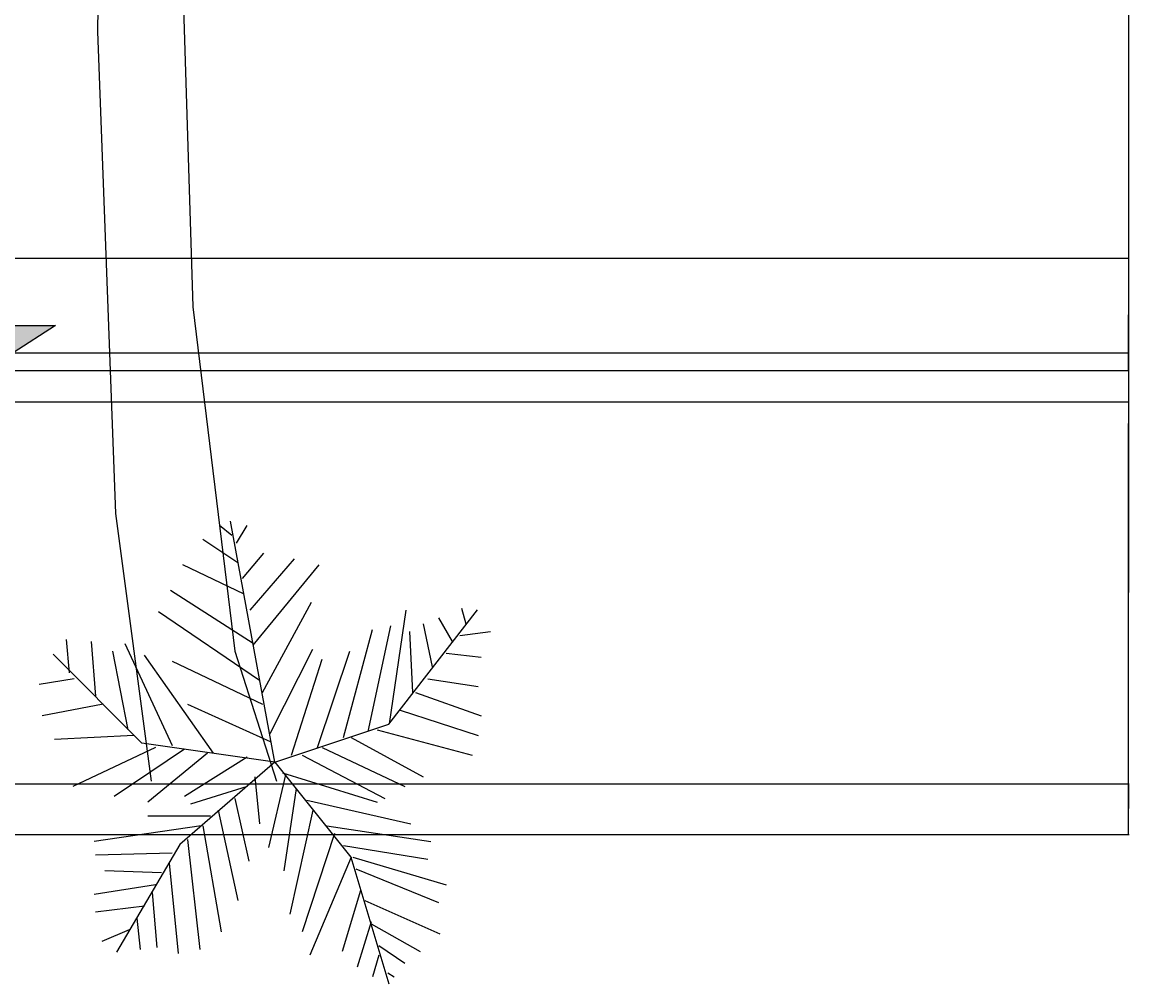
# Model space of a CAD drawing. Units: inches. Extents: x 484 to 1264, y 95 to 991.
# Tile 6 of 8: x 1002 to 1264, y 271 to 499. Entities that reach past the tile are written whole.
import ezdxf

# ---------------------------------------------------------------- set-up
doc = ezdxf.new("R2010")
doc.units = ezdxf.units.IN
doc.header["$MEASUREMENT"] = 0
doc.layers.add('A-ANNO-DIMS', color=2, linetype='Continuous', lineweight=18)
doc.layers.add('L-FENC', color=7, linetype='Continuous', lineweight=25)
doc.layers.add('A-ELEV-TRIM-PATT', color=40, linetype='Continuous', lineweight=13, true_color=0xe7c208)
doc.layers.add('TREES', color=92, linetype='Continuous')
doc.styles.get("Standard").update_dxf_attribs({"font": 'arial.ttf'})
doc.dimstyles.get("Standard").update_dxf_attribs({"dimtxt": 0.18, "dimasz": 0.18, "dimexe": 0.18, "dimexo": 0.0625, "dimgap": 0.09, "dimtad": 0, "dimtih": 1, "dimtoh": 1, "dimdec": 4, "dimzin": 0, "dimdsep": 46, "dimtxsty": 'Standard', "dimcen": 0.09, "dimadec": 0, "dimazin": 0, "dimtfac": 1, "dimtdec": 4, "dimtofl": 0, "dimtmove": 0, "dimatfit": 3, "dimfxl": 1, "dimtolj": 1, "dimtzin": 0, "dimarcsym": 0})

# ---------------------------------------------------------------- blocks, each defined once
blk = doc.blocks.new('*U2')
for p, q in [((-10.186, 53.64), (-13.084, 55.962)), ((0, 0), (-10.5, 57)), ((-9.099, 51.782), (-6.563, 55.962)), ((-8.737, 47.138), (-17.069, 52.711)), ((-7.65, 43.423), (-2.578, 49.46)), ((-5.839, 35.992), (4.667, 48.067)), ((-7.288, 39.707), (-21.778, 46.673)), ((-5.114, 27.632), (10.463, 46.673)), ((-5.114, 28.097), (-24.676, 40.636)), ((-2.941, 16.486), (8.652, 37.85)), ((-3.665, 19.273), (-27.574, 35.527)), ((27, 9), (48, 36)), ((27.127, 9.056), (31.112, 35.992)), ((38.719, 34.134), (41.979, 28.561)), ((44.153, 36.456), (45.239, 32.741)), ((22.055, 7.198), (27.489, 32.277)), ((35.096, 32.741), (37.27, 22.524)), ((-48.585, 21.131), (-49.309, 29.026)), ((16.259, 5.805), (23.142, 31.348)), ((31.836, 30.883), (32.561, 16.486)), ((43.791, 29.954), (51.036, 30.883)), ((-43.513, 28.561), (-42.427, 15.558)), ((-38.442, 26.239), (-34.819, 7.663)), ((-35.544, 28.097), (-24.314, 3.947)), ((-1.129, 6.734), (9.014, 26.704)), ((10.101, 3.483), (17.708, 26.239)), ((-31.5, 4.5), (-52.5, 25.5)), ((-14.533, 2.09), (-30.834, 25.31)), ((-24.314, 23.917), (-2.941, 13.7)), ((3.942, 1.625), (11.187, 24.381)), ((40.53, 25.775), (48.862, 24.846)), ((-47.498, 19.737), (-55.83, 18.344)), ((36.183, 19.737), (48.137, 17.88)), ((33.285, 16.486), (48.862, 10.913)), ((-40.615, 13.7), (-55.105, 10.913)), ((-20.691, 13.7), (-1.129, 4.876)), ((29.662, 12.307), (48.137, 6.269)), ((0, 0), (27, 9)), ((-33.37, 6.269), (-52.207, 5.34)), ((18.07, 5.805), (35.096, -3.483)), ((24.229, 7.663), (46.688, 1.625)), ((-28.299, 3.483), (-47.86, -5.805)), ((-21.416, 3.018), (-38.079, -8.128)), ((0, 0), (-31.5, 4.5)), ((11.187, 3.483), (30.749, -5.805)), ((-15.982, 2.09), (-30.11, -9.521)), ((0, 0), (-22.5, -19.5)), ((-6.563, 1.161), (-21.416, -8.128)), ((0, 0), (18, -22.5)), ((6.478, 1.625), (26.04, -8.592)), ((1.769, -2.555), (24.229, -9.521)), ((-4.752, -3.483), (-3.665, -14.629)), ((2.493, -3.019), (-1.491, -20.202)), ((-6.563, -5.805), (-19.967, -9.985)), ((5.029, -6.27), (2.131, -25.775)), ((-9.461, -8.592), (-6.201, -23.453)), ((7.565, -9.056), (32.198, -14.629)), ((-15.257, -12.772), (-30.11, -12.772)), ((-13.446, -11.378), (-8.737, -32.741)), ((9.014, -11.378), (3.58, -35.992)), ((-17.431, -15.094), (-42.789, -18.809)), ((-17.069, -15.094), (-12.721, -40.172)), ((12.274, -15.094), (36.907, -18.809)), ((-20.691, -18.345), (-17.793, -44.352)), ((14.085, -16.951), (6.478, -40.172)), ((-22.5, -19.5), (-37.5, -45)), ((16.259, -19.738), (36.183, -22.989)), ((-24.314, -21.596), (-42.427, -22.06)), ((18.07, -22.524), (8.289, -45.745)), ((18, -22.5), (27, -52.5)), ((18.433, -22.524), (40.53, -29.026)), ((-26.849, -26.24), (-40.253, -25.775)), ((-25.038, -23.918), (-22.865, -45.281)), ((19.157, -25.311), (38.719, -33.206)), ((-28.299, -29.026), (-42.789, -31.348)), ((-29.023, -30.884), (-27.936, -43.887)), ((20.244, -30.419), (15.897, -44.816)), ((21.331, -32.741), (39.081, -40.636)), ((-30.834, -34.135), (-42.427, -35.528)), ((-32.646, -36.921), (-31.921, -44.352)), ((22.78, -37.85), (19.519, -48.532)), ((22.78, -38.314), (34.372, -44.816)), ((-34.457, -39.708), (-40.978, -42.494)), ((24.591, -43.423), (30.749, -47.603)), ((24.591, -45.745), (23.142, -50.854)), ((26.764, -49.925), (28.213, -50.854))]:
    blk.add_line(p, q)
blk = doc.blocks.new('*U3')
for points in [[(-2.363, 170.553), (-3.88, 148.505), (-4.988, 69.634), (-3.325, 24.869), (0, 0)], [(-0.116, 162.848), (0.554, 143.532), (2.217, 96.635), (3.88, 44.054), (7.76, 12.079), (11.64, 0)]]:
    blk.add_lwpolyline(points)
blk = doc.blocks.new('FENCE-PIER-CAP')
for p, q in [((5.63, 0), (0, 6.48)), ((0, 6.48), (39.71, 6.48)), ((39.71, 6.48), (29.63, 0))]:
    blk.add_line(p, q)
blk = doc.blocks.new('*D18')
at = {"layer": 'A-ANNO-DIMS', "color": 0, "lineweight": -2, "transparency": 16777216}
for p, q in [((999.88, 501.38), (1264.08, 501.38)), ((1263.9, 501.2), (1263.9, 404.07)), ((1263.9, 306.56), (1263.9, 403.7)), ((595.38, 306.38), (1264.08, 306.38))]:
    blk.add_line(p, q, dxfattribs=at)
at = {"layer": 'A-ANNO-DIMS', "color": 0, "transparency": 16777216}
for points in [[(1263.87, 501.2), (1263.93, 501.2), (1263.9, 501.38)], [(1263.87, 306.56), (1263.93, 306.56), (1263.9, 306.38)]]:
    blk.add_solid(points, dxfattribs=at)
at = {"layer": 'Defpoints', "color": 0, "transparency": 16777216}
for p in [(999.81, 501.38), (1263.9, 501.38), (595.32, 306.38)]:
    blk.add_point(p, dxfattribs=at)
at = {"layer": 'A-ANNO-DIMS', "color": 0, "transparency": 16777216, "insert": (1263.9, 403.88), "char_height": 0.18, "attachment_point": 5}
blk.add_mtext('\\A1;195', dxfattribs=at)
blk = doc.blocks.new('*D50')
at = {"layer": 'A-ANNO-DIMS', "color": 0, "lineweight": -2, "transparency": 16777216}
for p, q in [((999.88, 420.38), (1264.08, 420.38)), ((1263.9, 420.2), (1263.9, 369.57)), ((1263.9, 318.56), (1263.9, 369.2)), ((999.88, 318.38), (1264.08, 318.38))]:
    blk.add_line(p, q, dxfattribs=at)
at = {"layer": 'A-ANNO-DIMS', "color": 0, "transparency": 16777216}
for points in [[(1263.87, 420.2), (1263.93, 420.2), (1263.9, 420.38)], [(1263.87, 318.56), (1263.93, 318.56), (1263.9, 318.38)]]:
    blk.add_solid(points, dxfattribs=at)
at = {"layer": 'Defpoints', "color": 0, "transparency": 16777216}
for p in [(999.81, 420.38), (1263.9, 420.38), (999.81, 318.38)]:
    blk.add_point(p, dxfattribs=at)
at = {"layer": 'A-ANNO-DIMS', "color": 0, "transparency": 16777216, "insert": (1263.9, 369.38), "char_height": 0.18, "attachment_point": 5}
blk.add_mtext('\\A1;102', dxfattribs=at)
blk = doc.blocks.new('*D56')
at = {"layer": 'A-ANNO-DIMS', "color": 0, "lineweight": -2, "transparency": 16777216}
for p, q in [((915.88, 408.78), (1264.08, 408.78)), ((1263.9, 408.6), (1263.9, 363.76)), ((1263.9, 318.56), (1263.9, 363.4)), ((915.88, 318.38), (1264.08, 318.38))]:
    blk.add_line(p, q, dxfattribs=at)
at = {"layer": 'A-ANNO-DIMS', "color": 0, "transparency": 16777216}
for points in [[(1263.87, 408.6), (1263.93, 408.6), (1263.9, 408.78)], [(1263.87, 318.56), (1263.93, 318.56), (1263.9, 318.38)]]:
    blk.add_solid(points, dxfattribs=at)
at = {"layer": 'Defpoints', "color": 0, "transparency": 16777216}
for p in [(915.81, 408.78), (1263.9, 408.78), (915.81, 318.38)]:
    blk.add_point(p, dxfattribs=at)
at = {"layer": 'A-ANNO-DIMS', "color": 0, "transparency": 16777216, "insert": (1263.9, 363.58), "char_height": 0.18, "attachment_point": 5}
blk.add_mtext('\\A1;90.4', dxfattribs=at)
blk = doc.blocks.new('*D59')
at = {"layer": 'A-ANNO-DIMS', "color": 0, "lineweight": -2, "transparency": 16777216}
for p, q in [((855.88, 318.38), (1264.08, 318.38)), ((1263.9, 318.2), (1263.9, 312.56)), ((1263.9, 306.56), (1263.9, 312.2)), ((855.88, 306.38), (1264.08, 306.38))]:
    blk.add_line(p, q, dxfattribs=at)
at = {"layer": 'A-ANNO-DIMS', "color": 0, "transparency": 16777216}
for points in [[(1263.87, 318.2), (1263.93, 318.2), (1263.9, 318.38)], [(1263.87, 306.56), (1263.93, 306.56), (1263.9, 306.38)]]:
    blk.add_solid(points, dxfattribs=at)
at = {"layer": 'Defpoints', "color": 0, "transparency": 16777216}
for p in [(855.81, 318.38), (855.81, 306.38), (1263.9, 306.38)]:
    blk.add_point(p, dxfattribs=at)
at = {"layer": 'A-ANNO-DIMS', "color": 0, "transparency": 16777216, "insert": (1263.9, 312.38), "char_height": 0.18, "attachment_point": 5}
blk.add_mtext('\\A1;12', dxfattribs=at)
blk = doc.blocks.new('*D62')
at = {"layer": 'A-ANNO-DIMS', "color": 0, "lineweight": -2, "transparency": 16777216}
for p, q in [((907.56, 442.78), (1264.08, 442.78)), ((1263.9, 442.6), (1263.9, 429.68)), ((1263.9, 416.4), (1263.9, 429.32)), ((907.18, 416.22), (1264.08, 416.22))]:
    blk.add_line(p, q, dxfattribs=at)
at = {"layer": 'A-ANNO-DIMS', "color": 0, "transparency": 16777216}
for points in [[(1263.87, 442.6), (1263.93, 442.6), (1263.9, 442.78)], [(1263.87, 416.4), (1263.93, 416.4), (1263.9, 416.22)]]:
    blk.add_solid(points, dxfattribs=at)
at = {"layer": 'Defpoints', "color": 0, "transparency": 16777216}
for p in [(907.5, 442.78), (907.12, 416.22), (1263.9, 416.22)]:
    blk.add_point(p, dxfattribs=at)
at = {"layer": 'A-ANNO-DIMS', "color": 0, "transparency": 16777216, "insert": (1263.9, 429.5), "char_height": 0.18, "attachment_point": 5}
blk.add_mtext('\\A1;26.56', dxfattribs=at)

msp = doc.modelspace()

# ---------------------------------------------------------------- hatches: boundary and pattern name
at = {"layer": 'A-ELEV-TRIM-PATT'}
h = msp.add_hatch(color=256, dxfattribs=at)
h.dxf.hatch_style = 1
h.paths.add_polyline_path([(629.3986, 426.86), (589.6936, 426.86), (595.3221, 420.3846), (619.3221, 420.3846)])
edge = h.paths.add_edge_path()
edge.add_line((857.8147, 421.9731), (857.8147, 421.9373))
edge.add_ellipse((838.7195, 429.7418), major_axis=(-35.8241, 0), ratio=0.25748145, start_angle=157.76958, end_angle=158.416192)
edge.add_line((858.2614, 422.011), (865.8912, 426.9141))
edge.add_line((865.8912, 426.9141), (826.1862, 426.9141))
edge.add_line((826.1862, 426.9141), (831.8617, 420.3846))
edge.add_line((831.8617, 420.3846), (855.7305, 420.3846))
edge.add_line((855.7305, 420.3846), (856.3445, 420.7792))
edge.add_line((856.3445, 420.7792), (857.8147, 421.9731))
h.paths.add_polyline_path([(1009.8912, 426.86), (970.1862, 426.86), (975.8147, 420.3846), (999.8147, 420.3846)])
h.paths.add_polyline_path([(857.8147, 421.7239), (856.3445, 420.7792), (855.8147, 420.3489), (855.8147, 396.3846), (857.8147, 396.3846)])
edge = h.paths.add_edge_path()
edge.add_ellipse((838.7195, 448.4615), major_axis=(-35.8241, 0), ratio=0.25748145, start_angle=154.631086, end_angle=157.76958, ccw=False)
edge.add_line((855.8147, 440.3555), (855.8147, 437.8478))
edge.add_ellipse((838.7195, 429.7418), major_axis=(-35.8241, 0), ratio=0.25748145, start_angle=202.23042, end_angle=205.368914, ccw=False)
edge.add_line((857.8147, 437.5462), (857.8147, 440.6571))
edge = h.paths.add_edge_path()
edge.add_line((907.4984, 442.7783), (866.9359, 442.7783))
edge.add_ellipse((838.7195, 448.4615), major_axis=(-35.8241, 0), ratio=0.25748145, start_angle=158.813461, end_angle=168.611984, ccw=False)
edge.add_line((858.542, 440.7783), (905.4984, 440.7783))
edge.add_line((905.4984, 440.7783), (905.4984, 418.7562))
edge.add_line((905.4984, 418.7562), (907.4984, 416.8218))
edge.add_line((907.4984, 416.8218), (907.4984, 442.7783))

# ---------------------------------------------------------------- block references
at = {"layer": 'L-FENC'}
msp.add_blockref('FENCE-PIER-CAP', (970.1862, 420.3846), dxfattribs=at)
at = {"layer": 'TREES', "xscale": 2.548367839539612, "yscale": 2.548367839539612, "zscale": 2.548367839539612}
msp.add_blockref('*U3', (1032.522, 319.0159), dxfattribs=at)
at = {"layer": 'TREES'}
msp.add_blockref('*U2', (1061.7984, 323.5306), dxfattribs=at)

# ---------------------------------------------------------------- dimensions: what is measured, and where the dimension line sits
at = {"layer": 'A-ANNO-DIMS'}
for base, p1, p2, override, picture, middle in [((1263.9032, 501.3846), (595.3221, 306.3846), (999.8147, 501.3846), {"dimdec": 0, "dimlfac": 1, "dimrnd": 0, "dimzin": 0, "dimdsep": 46, "dimlunit": 2}, '*D18', (1263.9032, 403.8846)), ((1263.9032, 416.2209), (907.4984, 442.7783), (907.1219, 416.2209), {"dimdec": 2, "dimlfac": 1, "dimrnd": 0, "dimzin": 0, "dimdsep": 46, "dimlunit": 2}, '*D62', (1263.9032, 429.4996)), ((1263.9032, 420.3846), (999.8147, 318.3846), (999.8147, 420.3846), {"dimdec": 0, "dimlfac": 1, "dimrnd": 0, "dimzin": 0, "dimdsep": 46, "dimlunit": 2}, '*D50', (1263.9032, 369.3846)), ((1263.9032, 408.7785), (915.8147, 318.3846), (915.8147, 408.7785), {"dimdec": 1, "dimlfac": 1, "dimrnd": 0, "dimzin": 0, "dimdsep": 46, "dimlunit": 2}, '*D56', (1263.9032, 363.5815)), ((1263.9032, 306.3846), (855.8147, 318.3846), (855.8147, 306.3846), {"dimdec": 0, "dimlfac": 1, "dimrnd": 0, "dimzin": 0, "dimdsep": 46, "dimlunit": 2}, '*D59', (1263.9032, 312.3846))]:
    dim = msp.add_linear_dim(base=base, p1=p1, p2=p2, angle=90, dimstyle='Standard', override=override, dxfattribs=at)
    dim.commit()
    dim.dimension.update_dxf_attribs({"geometry": picture, "text_midpoint": middle})

doc.saveas('drawing.dxf')
